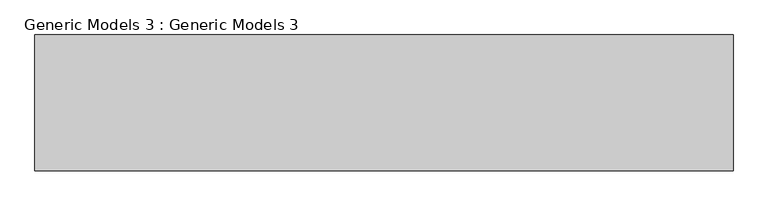
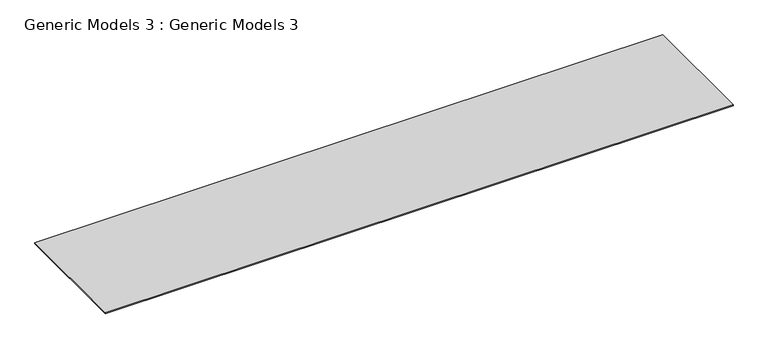
"""IFC4 building model written with IfcOpenShell, lengths in millimetres: proxy geometry, Generic Models 3 : Generic Models 3."""

from ifc_helpers import new_model, si_unit, frame, origin, place, context, project, spatial, polyline, outline, extrude, source, transform, mapped, element, save


def generic_models_3_generic_models_3_73c16d2e(model_context):
    return source(origin(), model_context, "Body", "SweptSolid", [
        extrude(outline(polyline([(13375.2014317, -18171.5677133), (-16109.2214715, -18171.5677133), (-16109.2214715, -12441.2064015), (13375.2014317, -12441.2064015), (13375.2014317, -18171.5677133)])), frame((0.0, 0.0, -609.6), z_axis=(0.0, 0.0, 1.0), x_axis=(1.0, 0.0, 0.0)), (0.0, 0.0, 1.0), 50.8),
    ])


if __name__ == "__main__":
    model = new_model("IFC4")
    model_context = context("Model", 3, world=origin())
    ifc_project = project(units=[si_unit("LENGTHUNIT", "METRE", prefix="MILLI")], contexts=[model_context])
    site = spatial("IfcSite", under=ifc_project)
    building = spatial("IfcBuilding", under=site)
    placement = place(None, origin())
    generic_models_3_generic_models_3_shape = generic_models_3_generic_models_3_73c16d2e(model_context)
    element("IfcBuildingElementProxy", 1, Name="Generic Models 3 : Generic Models 3", ObjectType="Generic Models 3 : Generic Models 3", at=placement, inside=building, context=model_context, shape_type="MappedRepresentation", body=[
        mapped(generic_models_3_generic_models_3_shape, transform((0.0, 0.0, 0.0), x_axis=(1.0, 0.0, 0.0), y_axis=(0.0, 1.0, 0.0), z_axis=(0.0, 0.0, 1.0))),
    ])
    save(model, "model.ifc")

# Revit data of these elements
# Element 1 (IfcBuildingElementProxy, "Generic Models 3 : Generic Models 3")
#   Materials on its faces: "SLAB"
# Materials
#   "SLAB": class "Generic", colour RGB 120 120 120, transparency 0, Cost = 0
